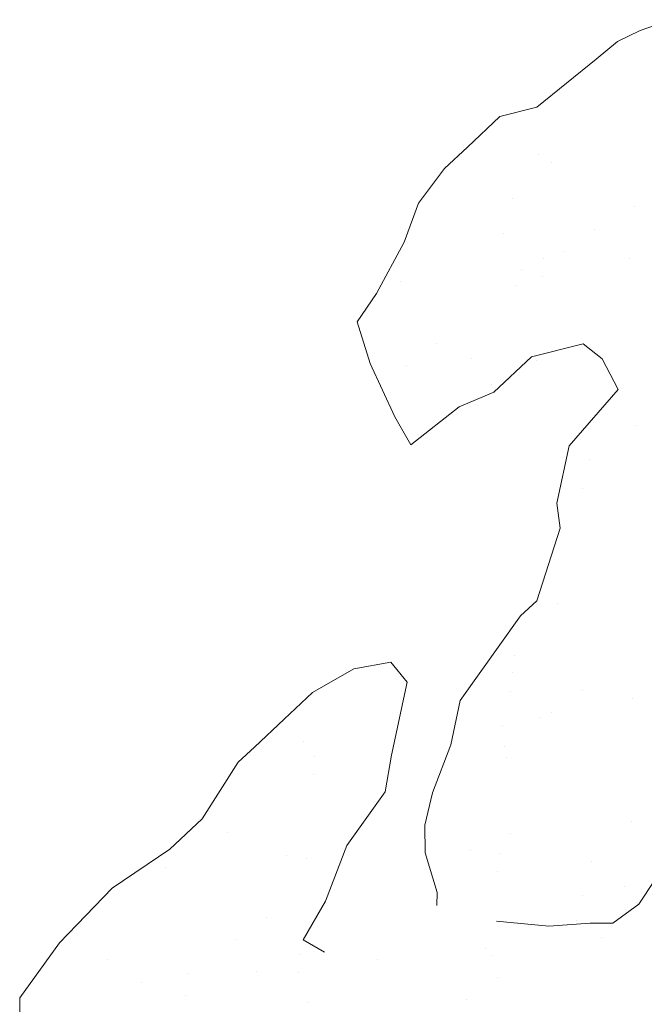
# Model space of a CAD drawing. Units: inches. Extents: x 1986 to 21484, y -1816 to 2016.
# Tile 59 of 85: x 3647.931 to 3651.423, y 1892.332 to 1897.834. Entities that reach past the tile are written whole.
import ezdxf

# ---------------------------------------------------------------- set-up
doc = ezdxf.new("R2010")
doc.units = ezdxf.units.IN
doc.layers.add('L-PLNT', color=84, linetype='Continuous', lineweight=13)

# ---------------------------------------------------------------- blocks, each defined once
blk = doc.blocks.new('PLANT-SHRUB')
for p, q in [((2170.5256, 1871.3679), (2170.6881, 1871.4058)), ((2170.6881, 1871.4058), (2170.8667, 1871.3842)), ((2170.8667, 1871.3842), (2170.9588, 1871.2976)), ((2170.9653, 1871.3971), (2170.9653, 1871.3971)), ((2170.6788, 1871.2788), (2170.6788, 1871.2788)), ((2170.9588, 1871.2976), (2171.1375, 1871.1515)), ((2171.0037, 1871.236), (2171.0037, 1871.236)), ((2170.886, 1871.1569), (2170.886, 1871.1569)), ((2171.1375, 1871.1515), (2171.3324, 1870.9297)), ((2171.5466, 1871.1645), (2171.5466, 1871.1645)), ((2171.7546, 1871.1372), (2171.7546, 1871.1372)), ((2170.4011, 1871.0406), (2170.4011, 1871.0406)), ((2170.7175, 1871.0495), (2170.7175, 1871.0495)), ((2171.4844, 1871.0503), (2171.4844, 1871.0503)), ((2171.4806, 1871.0017), (2171.4806, 1871.0017)), ((2171.1367, 1870.7317), (2171.1367, 1870.7317)), ((2171.063, 1870.6642), (2171.063, 1870.6642)), ((2170.9402, 1870.627), (2170.9402, 1870.627)), ((2171.5171, 1870.6384), (2171.4653, 1870.5867)), ((2171.9626, 1870.6319), (2171.9626, 1870.6319)), ((2169.9254, 1870.5448), (2169.9254, 1870.5448)), ((2171.17, 1870.5426), (2171.17, 1870.5426)), ((2171.4653, 1870.5867), (2171.3617, 1870.3797)), ((2172.4146, 1870.5403), (2172.4146, 1870.5403)), ((2171.3617, 1870.3797), (2171.2581, 1870.2658)), ((2172.1923, 1870.2675), (2172.1522, 1870.3993)), ((2172.3381, 1870.3809), (2172.3381, 1870.3809)), ((2170.1023, 1870.3199), (2170.1023, 1870.3199)), ((2172.2645, 1870.3134), (2172.2645, 1870.3134)), ((2170.3103, 1870.2925), (2170.3103, 1870.2925)), ((2170.376, 1870.2705), (2170.376, 1870.2705)), ((2170.6652, 1870.2997), (2170.6652, 1870.2997)), ((2171.2581, 1870.2658), (2171.1028, 1870.1623)), ((2171.9541, 1870.195), (2172.1923, 1870.2675)), ((2172.1923, 1870.2675), (2172.1923, 1870.2675)), ((2170.6352, 1870.2497), (2170.6352, 1870.2497)), ((2172.5016, 1870.2183), (2172.5016, 1870.2183)), ((2170.5632, 1870.156), (2170.5632, 1870.156)), ((2171.1028, 1870.1623), (2170.8439, 1870.0382)), ((2171.6537, 1870.0501), (2171.9541, 1870.195)), ((2170.3947, 1870.0487), (2170.3947, 1870.0487)), ((2170.8439, 1870.0382), (2170.6367, 1869.8933)), ((2171.2912, 1869.9777), (2171.6537, 1870.0501)), ((2171.6393, 1870.0464), (2171.6393, 1870.0464)), ((2171.6537, 1870.0501), (2171.6537, 1870.0501)), ((2172.884, 1870.0441), (2172.884, 1870.0441)), ((2172.2539, 1870.0366), (2172.2539, 1870.0366)), ((2172.4619, 1870.0092), (2172.4619, 1870.0092)), ((2170.3175, 1869.9811), (2170.3175, 1869.9811)), ((2171.1255, 1869.8535), (2171.2912, 1869.9777)), ((2171.8667, 1869.9489), (2171.8667, 1869.9489)), ((2172.7869, 1869.9664), (2172.7869, 1869.9664)), ((2170.6367, 1869.8933), (2170.0671, 1869.7794)), ((2170.2438, 1869.9136), (2170.2438, 1869.9136)), ((2169.8688, 1869.8702), (2169.8688, 1869.8702)), ((2170.7837, 1869.6155), (2171.1255, 1869.8535)), ((2171.1255, 1869.8535), (2171.1255, 1869.8535)), ((2171.9374, 1869.8618), (2171.9374, 1869.8618)), ((2173.0169, 1869.8229), (2173.0169, 1869.8229)), ((2169.9428, 1869.7794), (2169.5699, 1869.5724)), ((2170.0671, 1869.7794), (2169.9428, 1869.7794)), ((2170.7733, 1869.4706), (2170.7837, 1869.6155)), ((2171.519, 1869.6303), (2171.519, 1869.6303)), ((2173.0681, 1869.5981), (2173.0681, 1869.5981)), ((2169.5699, 1869.5724), (2169.4871, 1869.4586)), ((2171.4453, 1869.5628), (2171.4453, 1869.5628)), ((2173.6837, 1869.543), (2173.5698, 1869.4188)), ((2169.3284, 1869.4955), (2169.3284, 1869.4955)), ((2172.0918, 1869.5395), (2172.0918, 1869.5395)), ((2168.866, 1869.4478), (2168.866, 1869.4478)), ((2169.4871, 1869.4586), (2169.2178, 1869.2723)), ((2169.4871, 1869.4586), (2169.4871, 1869.4586)), ((2170.9494, 1869.3567), (2170.7733, 1869.4706)), ((2171.4302, 1869.4615), (2171.4302, 1869.4615)), ((2172.4764, 1869.4482), (2172.4764, 1869.4482)), ((2169.1909, 1869.4051), (2169.1909, 1869.4051)), ((2172.1405, 1869.3878), (2171.778, 1869.2946)), ((2172.3891, 1869.3878), (2172.1405, 1869.3878)), ((2172.7723, 1869.3257), (2172.3891, 1869.3878)), ((2173.5698, 1869.4188), (2173.1969, 1869.3464)), ((2171.2083, 1869.2946), (2170.9494, 1869.3567)), ((2173.1969, 1869.3464), (2172.7723, 1869.3257)), ((2172.7723, 1869.3257), (2172.7723, 1869.3257)), ((2173.1969, 1869.3464), (2173.1969, 1869.3464)), ((2169.2178, 1869.2723), (2168.8035, 1869.2309)), ((2171.4258, 1869.2946), (2171.2083, 1869.2946)), ((2171.4258, 1869.2946), (2171.4258, 1869.2946)), ((2171.6537, 1869.2946), (2171.4258, 1869.2946)), ((2171.778, 1869.2946), (2171.6537, 1869.2946)), ((2168.8035, 1869.2309), (2168.7517, 1869.0446)), ((2168.8035, 1869.2309), (2168.8035, 1869.2309)), ((2168.7517, 1869.0446), (2168.7724, 1868.9101)), ((2168.7724, 1868.9101), (2169.0313, 1868.7652)), ((2168.7724, 1868.9101), (2168.7724, 1868.9101)), ((2169.0269, 1868.7984), (2169.0269, 1868.7984)), ((2168.257, 1868.7388), (2168.257, 1868.7388)), ((2169.0313, 1868.7652), (2169.3213, 1868.7652)), ((2169.3032, 1868.7254), (2169.3032, 1868.7254)), ((2169.3213, 1868.7652), (2169.5181, 1868.6928)), ((2169.5181, 1868.6928), (2169.8599, 1868.6617)), ((2169.5181, 1868.6928), (2169.5181, 1868.6928)), ((2169.8599, 1868.6617), (2169.8185, 1868.4858)), ((2168.0351, 1868.5455), (2168.0351, 1868.5455)), ((2169.2798, 1868.5432), (2169.2798, 1868.5432)), ((2168.2894, 1868.4889), (2168.2894, 1868.4889)), ((2168.4975, 1868.4615), (2168.4975, 1868.4615)), ((2168.6791, 1868.4798), (2168.6791, 1868.4798)), ((2169.8185, 1868.4858), (2169.7149, 1868.1753)), ((2169.8185, 1868.4858), (2169.8185, 1868.4858)), ((2168.6055, 1868.4123), (2168.6055, 1868.4123)), ((2168.8224, 1868.4188), (2168.8224, 1868.4188)), ((2168.739, 1868.3689), (2168.739, 1868.3689)), ((2169.3653, 1868.3473), (2169.3653, 1868.3473)), ((2169.5733, 1868.3199), (2169.5733, 1868.3199)), ((2169.7149, 1868.1753), (2169.6088, 1867.9557)), ((2168.673, 1868.1567), (2168.673, 1868.1567)), ((2168.2077, 1868.0478), (2168.2077, 1868.0478)), ((2168.5045, 1868.0493), (2168.5045, 1868.0493)), ((2168.2319, 1867.9687), (2168.2319, 1867.9687)), ((2169.278, 1867.9553), (2169.278, 1867.9553)), ((2169.6088, 1867.9557), (2169.4224, 1867.9143)), ((2167.3406, 1867.8522), (2167.1749, 1867.9247)), ((2169.4224, 1867.9143), (2169.1117, 1867.8108)), ((2169.4224, 1867.9143), (2169.4224, 1867.9143)), ((2167.4752, 1867.8108), (2167.3406, 1867.8522)), ((2167.6306, 1867.8005), (2167.4752, 1867.8108)), ((2168.0552, 1867.7695), (2167.6306, 1867.8005)), ((2169.1117, 1867.8108), (2168.9045, 1867.7074)), ((2168.2417, 1867.666), (2168.0552, 1867.7695)), ((2168.9045, 1867.7074), (2168.6663, 1867.666)), ((2168.4902, 1867.666), (2168.2417, 1867.666)), ((2168.6663, 1867.666), (2168.4902, 1867.666))]:
    blk.add_line(p, q)

msp = doc.modelspace()

# ---------------------------------------------------------------- block references
at = {"layer": 'L-PLNT', "rotation": 223.1883365522388}
msp.add_blockref('PLANT-SHRUB', (3953.27, 4742.9646), dxfattribs=at)

doc.saveas('drawing.dxf')
